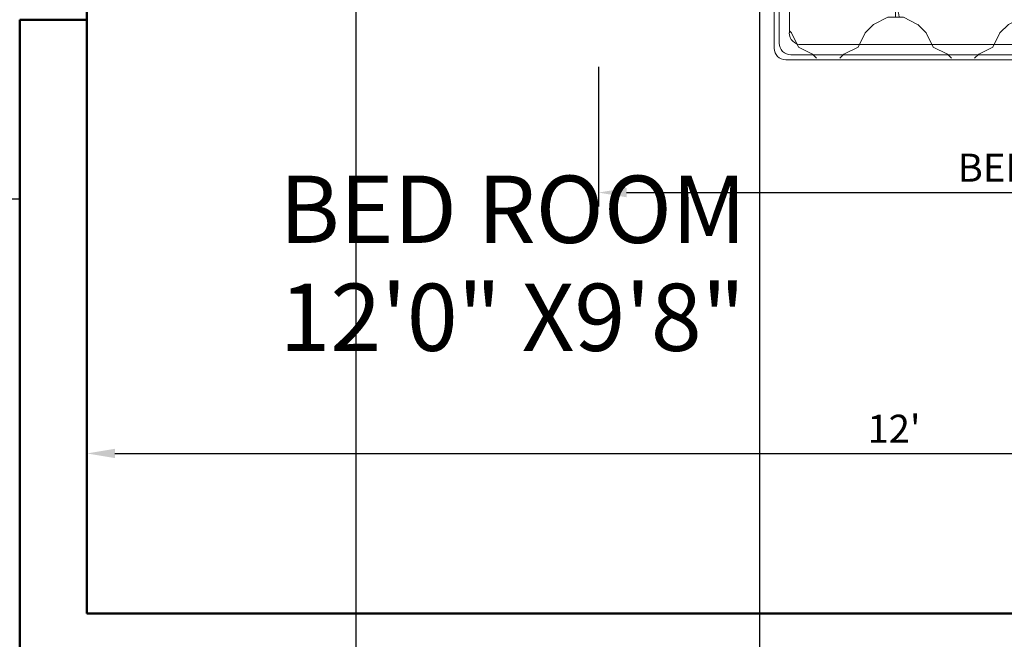
# Model space of a CAD drawing. Units: inches. Extents: x 2385 to 2740, y 1752 to 2305.
# Tile 3 of 15: x 2553 to 2641, y 1861 to 1916. Entities that reach past the tile are written whole.
import ezdxf

# ---------------------------------------------------------------- set-up
doc = ezdxf.new("R2010")
doc.units = ezdxf.units.IN
for name, color, linetype, lineweight in [('A-ANNO-DIMS', 2, 'Continuous', 18), ('A-AREA-IDEN', 7, 'Continuous', 25), ('A-FLOR-STRS', 7, 'Continuous', 25), ('A-FURN', 9, 'Continuous', 18), ('A-WALL', 7, 'Continuous', 50)]:
    doc.layers.add(name, color=color, linetype=linetype, lineweight=lineweight)
doc.styles.get("Standard").update_dxf_attribs({"font": 'arial.ttf'})
doc.dimstyles.new('Copy of ISO-25', dxfattribs={"dimtxt": 2.5, "dimasz": 2.5, "dimexe": 1.25, "dimexo": 0.625, "dimtad": 1, "dimdec": 1, "dimlunit": 4, "dimtxsty": 'Standard', "dimcen": 2.5, "dimadec": 0, "dimazin": 0, "dimtfac": 1, "dimtdec": 1, "dimtmove": 0, "dimatfit": 3, "dimfxl": 1, "dimarcsym": 0})

# ---------------------------------------------------------------- blocks, each defined once
blk = doc.blocks.new('A$C029D5C69')
for p, q in [((0.4164, 2.0693), (0.4164, 2.0066)), ((2.2315, 2.0693), (0.4164, 2.0693)), ((2.2315, 2.0066), (2.2315, 2.0693)), ((0, 1.606), (0, 2.0066)), ((0, 2.0066), (0.505, 2.0066)), ((0.4164, 2.0066), (2.2315, 2.0066)), ((0.505, 2.0066), (0.505, 1.606)), ((0.5252, 0.0351), (0.5252, 2.0066)), ((0.5403, 0.0502), (0.5403, 2.0066)), ((0.5706, 0.0805), (0.5706, 2.0066)), ((0.6869, 1.966), (0.6666, 2.0066)), ((0.7072, 2.0066), (0.6869, 1.966)), ((1.0902, 1.966), (1.0699, 2.0066)), ((1.1106, 2.0066), (1.0902, 1.966)), ((2.1114, 2.0087), (2.1114, 0.0351)), ((2.6479, 2.0066), (2.1429, 2.0066)), ((2.1429, 2.0066), (2.1429, 1.606)), ((2.6479, 1.606), (2.6479, 2.0066)), ((0.0151, 1.6211), (0.0151, 1.9915)), ((0.0151, 1.9915), (0.4899, 1.9915)), ((0.4899, 1.9915), (0.4899, 1.6211)), ((1.8954, 1.9865), (1.3081, 1.9865)), ((2.6328, 1.9915), (2.158, 1.9915)), ((2.158, 1.9915), (2.158, 1.6211)), ((2.6328, 1.6211), (2.6328, 1.9915)), ((0.2689, 1.9609), (0.2689, 1.6764)), ((0.6869, 1.9425), (0.6869, 1.966)), ((0.6869, 1.9425), (0.6869, 1.966)), ((1.0902, 1.9425), (1.0902, 1.966)), ((1.0902, 1.9425), (1.0902, 1.966)), ((1.8954, 1.9713), (1.3339, 1.9713)), ((1.3849, 1.9713), (1.3656, 1.952)), ((1.3945, 1.9713), (1.3714, 1.9483)), ((1.4249, 1.945), (1.3986, 1.9713)), ((1.4249, 1.945), (1.4059, 1.926)), ((1.4288, 1.9507), (1.4081, 1.9713)), ((1.4476, 1.9507), (1.4288, 1.9507)), ((1.4476, 1.9507), (1.4664, 1.9507)), ((1.487, 1.9713), (1.4664, 1.9507)), ((1.4966, 1.9713), (1.4703, 1.945)), ((1.4986, 1.9167), (1.4703, 1.945)), ((1.527, 1.945), (1.4986, 1.9167)), ((1.527, 1.945), (1.5007, 1.9713)), ((1.5309, 1.9507), (1.5102, 1.9713)), ((1.5497, 1.9507), (1.5309, 1.9507)), ((1.5497, 1.9507), (1.5685, 1.9507)), ((1.5891, 1.9713), (1.5685, 1.9507)), ((1.5987, 1.9713), (1.5724, 1.945)), ((1.6007, 1.9167), (1.5724, 1.945)), ((1.6291, 1.945), (1.6007, 1.9167)), ((1.6291, 1.945), (1.6028, 1.9713)), ((1.633, 1.9507), (1.6123, 1.9713)), ((1.6518, 1.9507), (1.633, 1.9507)), ((1.6518, 1.9507), (1.6706, 1.9507)), ((1.6912, 1.9713), (1.6706, 1.9507)), ((1.7008, 1.9713), (1.6745, 1.945)), ((1.7028, 1.9167), (1.6745, 1.945)), ((1.7312, 1.945), (1.7028, 1.9167)), ((1.7312, 1.945), (1.7049, 1.9713)), ((1.7351, 1.9507), (1.7144, 1.9713)), ((1.7539, 1.9507), (1.7351, 1.9507)), ((1.7539, 1.9507), (1.7727, 1.9507)), ((1.7933, 1.9713), (1.7727, 1.9507)), ((1.8029, 1.9713), (1.7766, 1.945)), ((1.8049, 1.9167), (1.7766, 1.945)), ((1.8333, 1.945), (1.8049, 1.9167)), ((1.8333, 1.945), (1.807, 1.9713)), ((1.8372, 1.9507), (1.8165, 1.9713)), ((1.856, 1.9507), (1.8372, 1.9507)), ((1.856, 1.9507), (1.8748, 1.9507)), ((1.8954, 1.9713), (1.8748, 1.9507)), ((1.9043, 1.9707), (1.8787, 1.945)), ((1.907, 1.9167), (1.8787, 1.945)), ((1.9354, 1.945), (1.907, 1.9167)), ((1.9354, 1.945), (1.9114, 1.969)), ((2.379, 1.9609), (2.379, 1.6764)), ((0.621, 1.9213), (0.5955, 1.8958)), ((0.6634, 1.9425), (0.621, 1.9213)), ((0.6634, 1.9425), (0.621, 1.9213)), ((0.6869, 1.9425), (0.6634, 1.9425)), ((0.6869, 1.9425), (0.7104, 1.9425)), ((0.7528, 1.9213), (0.7104, 1.9425)), ((0.7528, 1.9213), (0.7104, 1.9425)), ((0.7783, 1.8958), (0.7528, 1.9213)), ((1.0243, 1.9213), (0.9988, 1.8958)), ((1.0668, 1.9425), (1.0244, 1.9213)), ((1.0668, 1.9425), (1.0244, 1.9213)), ((1.0902, 1.9425), (1.0668, 1.9425)), ((1.0902, 1.9425), (1.1137, 1.9425)), ((1.1561, 1.9213), (1.1137, 1.9425)), ((1.1561, 1.9213), (1.1137, 1.9425)), ((1.1816, 1.8958), (1.1561, 1.9213)), ((1.4288, 1.9394), (1.4116, 1.9222)), ((1.4288, 1.9393), (1.4476, 1.9393)), ((1.4664, 1.9393), (1.4476, 1.9393)), ((1.493, 1.9128), (1.4664, 1.9394)), ((1.5309, 1.9394), (1.5043, 1.9128)), ((1.5309, 1.9393), (1.5497, 1.9393)), ((1.5685, 1.9393), (1.5497, 1.9393)), ((1.595, 1.9128), (1.5685, 1.9394)), ((1.633, 1.9394), (1.6064, 1.9128)), ((1.633, 1.9393), (1.6518, 1.9393)), ((1.6706, 1.9393), (1.6518, 1.9393)), ((1.6971, 1.9128), (1.6706, 1.9394)), ((1.7351, 1.9394), (1.7085, 1.9128)), ((1.7351, 1.9393), (1.7539, 1.9393)), ((1.7727, 1.9393), (1.7539, 1.9393)), ((1.7992, 1.9128), (1.7727, 1.9394)), ((1.8372, 1.9394), (1.8106, 1.9128)), ((1.8372, 1.9393), (1.856, 1.9393)), ((1.8748, 1.9393), (1.856, 1.9393)), ((1.9013, 1.9128), (1.8748, 1.9394)), ((1.9393, 1.9394), (1.9127, 1.9128)), ((1.9393, 1.9393), (1.9404, 1.9393)), ((1.9414, 1.688), (1.9414, 1.931)), ((1.9565, 1.688), (1.9565, 1.931)), ((0.5955, 1.8958), (0.5743, 1.8534)), ((0.7995, 1.8534), (0.7783, 1.8958)), ((0.9989, 1.8958), (0.9777, 1.8534)), ((1.2028, 1.8534), (1.1816, 1.8958)), ((1.493, 1.8752), (1.493, 1.9128)), ((1.5043, 1.8752), (1.5043, 1.9128)), ((1.595, 1.8752), (1.595, 1.9128)), ((1.6064, 1.8752), (1.6064, 1.9128)), ((1.6971, 1.8752), (1.6971, 1.9128)), ((1.7085, 1.8752), (1.7085, 1.9128)), ((1.7992, 1.8752), (1.7992, 1.9128)), ((1.8106, 1.8752), (1.8106, 1.9128)), ((1.9013, 1.8752), (1.9013, 1.9128)), ((1.9127, 1.8752), (1.9127, 1.9128)), ((1.493, 1.8752), (1.4867, 1.869)), ((1.4986, 1.8713), (1.4922, 1.8648)), ((1.527, 1.8429), (1.4986, 1.8713)), ((1.5309, 1.8486), (1.5043, 1.8752)), ((1.595, 1.8752), (1.5685, 1.8486)), ((1.6007, 1.8713), (1.5724, 1.8429)), ((1.6291, 1.8429), (1.6007, 1.8713)), ((1.633, 1.8486), (1.6064, 1.8752)), ((1.6971, 1.8752), (1.6706, 1.8486)), ((1.7028, 1.8713), (1.6745, 1.8429)), ((1.7312, 1.8429), (1.7028, 1.8713)), ((1.7351, 1.8486), (1.7085, 1.8752)), ((1.7992, 1.8752), (1.7727, 1.8486)), ((1.8049, 1.8713), (1.7766, 1.8429)), ((1.8333, 1.8429), (1.8049, 1.8713)), ((1.8372, 1.8486), (1.8106, 1.8752)), ((1.9013, 1.8752), (1.8748, 1.8486)), ((1.907, 1.8713), (1.8787, 1.8429)), ((1.9354, 1.8429), (1.907, 1.8713)), ((1.9393, 1.8486), (1.9127, 1.8752)), ((0.5743, 1.8534), (0.5706, 1.8515)), ((0.5743, 1.8534), (0.5706, 1.8515)), ((0.8419, 1.8322), (0.7995, 1.8534)), ((0.8419, 1.8322), (0.7995, 1.8534)), ((0.8674, 1.8067), (0.8419, 1.8322)), ((0.9352, 1.8322), (0.9097, 1.8067)), ((0.9777, 1.8534), (0.9353, 1.8322)), ((0.9777, 1.8534), (0.9353, 1.8322)), ((1.2452, 1.8322), (1.2028, 1.8534)), ((1.2452, 1.8322), (1.2028, 1.8534)), ((1.2707, 1.8067), (1.2452, 1.8322)), ((1.527, 1.8429), (1.5242, 1.8401)), ((1.5309, 1.8373), (1.5295, 1.8359)), ((1.5497, 1.8486), (1.5309, 1.8486)), ((1.5309, 1.8373), (1.5497, 1.8373)), ((1.5497, 1.8486), (1.5685, 1.8486)), ((1.5685, 1.8373), (1.5497, 1.8373)), ((1.595, 1.8107), (1.5685, 1.8373)), ((1.6007, 1.8146), (1.5724, 1.8429)), ((1.6291, 1.8429), (1.6007, 1.8146)), ((1.633, 1.8373), (1.6064, 1.8107)), ((1.6518, 1.8486), (1.633, 1.8486)), ((1.633, 1.8373), (1.6518, 1.8373)), ((1.6518, 1.8486), (1.6706, 1.8486)), ((1.6706, 1.8373), (1.6518, 1.8373)), ((1.6971, 1.8107), (1.6706, 1.8373)), ((1.7028, 1.8146), (1.6745, 1.8429)), ((1.7312, 1.8429), (1.7028, 1.8146)), ((1.7351, 1.8373), (1.7085, 1.8107)), ((1.7539, 1.8486), (1.7351, 1.8486)), ((1.7351, 1.8373), (1.7539, 1.8373)), ((1.7539, 1.8486), (1.7727, 1.8486)), ((1.7727, 1.8373), (1.7539, 1.8373)), ((1.7992, 1.8107), (1.7727, 1.8373)), ((1.8049, 1.8146), (1.7766, 1.8429)), ((1.8333, 1.8429), (1.8049, 1.8146)), ((1.8372, 1.8373), (1.8106, 1.8107)), ((1.856, 1.8486), (1.8372, 1.8486)), ((1.8372, 1.8373), (1.856, 1.8373)), ((1.856, 1.8486), (1.8748, 1.8486)), ((1.8748, 1.8373), (1.856, 1.8373)), ((1.9013, 1.8107), (1.8748, 1.8373)), ((1.907, 1.8146), (1.8787, 1.8429)), ((1.9354, 1.8429), (1.907, 1.8146)), ((1.9393, 1.8373), (1.9127, 1.8107)), ((1.9414, 1.8486), (1.9393, 1.8486)), ((1.9393, 1.8373), (1.9414, 1.8373)), ((0.1267, 1.8186), (0.4111, 1.8186)), ((0.8886, 1.7643), (0.8674, 1.8067)), ((0.9098, 1.8067), (0.8886, 1.7643)), ((1.2919, 1.7643), (1.2707, 1.8067)), ((1.595, 1.7806), (1.595, 1.8107)), ((1.6064, 1.7731), (1.6064, 1.8107)), ((1.6971, 1.7731), (1.6971, 1.8107)), ((1.7085, 1.7731), (1.7085, 1.8107)), ((1.7992, 1.7731), (1.7992, 1.8107)), ((1.8106, 1.7731), (1.8106, 1.8107)), ((1.9013, 1.7731), (1.9013, 1.8107)), ((1.9127, 1.7731), (1.9127, 1.8107)), ((2.2367, 1.8186), (2.5212, 1.8186)), ((1.2981, 1.7768), (1.2919, 1.7643)), ((1.633, 1.7465), (1.6064, 1.7731)), ((1.6971, 1.7731), (1.6706, 1.7465)), ((1.7028, 1.7692), (1.6745, 1.7408)), ((1.7312, 1.7408), (1.7028, 1.7692)), ((1.7351, 1.7465), (1.7085, 1.7731)), ((1.7992, 1.7731), (1.7727, 1.7465)), ((1.8049, 1.7692), (1.7766, 1.7408)), ((1.8333, 1.7408), (1.8049, 1.7692)), ((1.8372, 1.7465), (1.8106, 1.7731)), ((1.9013, 1.7731), (1.8748, 1.7465)), ((1.907, 1.7692), (1.8787, 1.7408)), ((1.9354, 1.7408), (1.907, 1.7692)), ((1.9393, 1.7465), (1.9127, 1.7731)), ((0.8651, 1.7408), (0.8227, 1.7196)), ((0.8651, 1.7408), (0.8227, 1.7196)), ((0.912, 1.7408), (0.8651, 1.7408)), ((0.8886, 1.7408), (0.8886, 1.7643)), ((0.9544, 1.7196), (0.912, 1.7408)), ((0.9544, 1.7196), (0.912, 1.7408)), ((1.2684, 1.7408), (1.226, 1.7196)), ((1.2684, 1.7408), (1.226, 1.7196)), ((1.2885, 1.7408), (1.2684, 1.7408)), ((1.2919, 1.7519), (1.2919, 1.7643)), ((1.6518, 1.7465), (1.633, 1.7465)), ((1.6518, 1.7465), (1.6706, 1.7465)), ((1.7028, 1.7125), (1.6745, 1.7408)), ((1.7312, 1.7408), (1.7028, 1.7125)), ((1.7539, 1.7465), (1.7351, 1.7465)), ((1.7539, 1.7465), (1.7727, 1.7465)), ((1.8049, 1.7125), (1.7766, 1.7408)), ((1.8333, 1.7408), (1.8049, 1.7125)), ((1.856, 1.7465), (1.8372, 1.7465)), ((1.856, 1.7465), (1.8748, 1.7465)), ((1.907, 1.7125), (1.8787, 1.7408)), ((1.9354, 1.7408), (1.907, 1.7125)), ((1.9414, 1.7465), (1.9393, 1.7465)), ((0.8227, 1.7196), (0.7972, 1.6941)), ((0.98, 1.6941), (0.9545, 1.7196)), ((1.226, 1.7196), (1.2005, 1.6941)), ((1.6443, 1.7352), (1.6518, 1.7352)), ((1.6706, 1.7352), (1.6518, 1.7352)), ((1.6971, 1.7086), (1.6706, 1.7352)), ((1.6971, 1.682), (1.6971, 1.7086)), ((1.7351, 1.7352), (1.7085, 1.7086)), ((1.7085, 1.671), (1.7085, 1.7086)), ((1.7351, 1.7352), (1.7539, 1.7352)), ((1.7727, 1.7352), (1.7539, 1.7352)), ((1.7992, 1.7086), (1.7727, 1.7352)), ((1.7992, 1.671), (1.7992, 1.7086)), ((1.8372, 1.7352), (1.8106, 1.7086)), ((1.8106, 1.671), (1.8106, 1.7086)), ((1.8372, 1.7352), (1.856, 1.7352)), ((1.8748, 1.7352), (1.856, 1.7352)), ((1.9013, 1.7086), (1.8748, 1.7352)), ((1.9013, 1.671), (1.9013, 1.7086)), ((1.9393, 1.7352), (1.9127, 1.7086)), ((1.9127, 1.671), (1.9127, 1.7086)), ((1.9393, 1.7352), (1.9414, 1.7352)), ((0.5766, 1.6941), (0.5706, 1.7002)), ((0.5978, 1.6517), (0.5766, 1.6941)), ((0.7972, 1.6941), (0.776, 1.6517)), ((1.0011, 1.6517), (0.9799, 1.6941)), ((1.2005, 1.6941), (1.1793, 1.6517)), ((2.5551, 1.6275), (2.5551, 1.696)), ((0.6402, 1.6305), (0.5978, 1.6517)), ((0.6402, 1.6305), (0.5978, 1.6517)), ((0.776, 1.6517), (0.7336, 1.6305)), ((0.776, 1.6517), (0.7336, 1.6305)), ((1.0435, 1.6305), (1.0011, 1.6517)), ((1.0435, 1.6305), (1.0011, 1.6517)), ((1.1793, 1.6517), (1.1369, 1.6305)), ((1.1793, 1.6517), (1.1369, 1.6305)), ((1.7318, 1.6477), (1.7085, 1.671)), ((1.7992, 1.671), (1.7759, 1.6477)), ((1.8049, 1.6671), (1.7855, 1.6477)), ((1.8244, 1.6477), (1.8049, 1.6671)), ((1.8339, 1.6477), (1.8106, 1.671)), ((1.9013, 1.671), (1.878, 1.6477)), ((1.907, 1.6671), (1.8876, 1.6477)), ((1.9202, 1.6539), (1.907, 1.6671)), ((1.926, 1.6577), (1.9127, 1.671)), ((0.4899, 1.6211), (0.0151, 1.6211)), ((0.6657, 1.605), (0.6402, 1.6305)), ((0.7336, 1.6305), (0.7081, 1.605)), ((1.0691, 1.605), (1.0436, 1.6305)), ((1.1369, 1.6305), (1.1114, 1.605)), ((1.8961, 1.6477), (1.7289, 1.6477)), ((1.8961, 1.6325), (1.7422, 1.6325)), ((2.158, 1.6211), (2.6328, 1.6211)), ((0.505, 1.606), (0, 1.606)), ((0.6869, 1.5626), (0.6657, 1.605)), ((0.7081, 1.605), (0.6869, 1.5626)), ((1.0902, 1.5626), (1.069, 1.605)), ((1.1114, 1.605), (1.0902, 1.5626)), ((2.1429, 1.606), (2.6479, 1.606)), ((0.6869, 1.5392), (0.6869, 1.5626)), ((0.6869, 1.5392), (0.6869, 1.5626)), ((1.0902, 1.5392), (1.0902, 1.5626)), ((1.0902, 1.5392), (1.0902, 1.5626)), ((0.6634, 1.5391), (0.621, 1.5179)), ((0.6634, 1.5391), (0.621, 1.5179)), ((0.6869, 1.5392), (0.6634, 1.5392)), ((0.6869, 1.5392), (0.7104, 1.5392)), ((0.7528, 1.5179), (0.7104, 1.5391)), ((0.7528, 1.5179), (0.7104, 1.5391)), ((1.0668, 1.5391), (1.0244, 1.5179)), ((1.0668, 1.5391), (1.0244, 1.5179)), ((1.0902, 1.5392), (1.0668, 1.5392)), ((1.0902, 1.5392), (1.1137, 1.5392)), ((1.1561, 1.5179), (1.1137, 1.5391)), ((1.1561, 1.5179), (1.1137, 1.5391)), ((0.621, 1.5179), (0.5955, 1.4924)), ((0.7783, 1.4924), (0.7528, 1.5179)), ((1.0243, 1.5179), (0.9988, 1.4924)), ((1.1816, 1.4924), (1.1561, 1.5179)), ((1.4277, 1.5179), (1.4022, 1.4924)), ((1.4534, 1.5308), (1.4277, 1.5179)), ((1.4534, 1.5308), (1.4277, 1.5179)), ((0.5955, 1.4925), (0.5743, 1.4501)), ((0.7995, 1.4501), (0.7783, 1.4925)), ((0.9989, 1.4925), (0.9777, 1.4501)), ((1.2028, 1.4501), (1.1816, 1.4925)), ((1.4022, 1.4925), (1.381, 1.4501)), ((0.5743, 1.45), (0.5706, 1.4481)), ((0.5743, 1.45), (0.5706, 1.4481)), ((0.8419, 1.4288), (0.7995, 1.45)), ((0.8419, 1.4288), (0.7995, 1.45)), ((0.9777, 1.45), (0.9353, 1.4288)), ((0.9777, 1.45), (0.9353, 1.4288)), ((1.2452, 1.4288), (1.2028, 1.45)), ((1.2452, 1.4288), (1.2028, 1.45)), ((1.381, 1.45), (1.3386, 1.4288)), ((1.381, 1.45), (1.3386, 1.4288)), ((1.6062, 1.4501), (1.5966, 1.4692)), ((1.6486, 1.4288), (1.6062, 1.45)), ((1.6486, 1.4288), (1.6062, 1.45)), ((0.8674, 1.4033), (0.8419, 1.4288)), ((0.9352, 1.4288), (0.9097, 1.4033)), ((1.2707, 1.4033), (1.2452, 1.4288)), ((1.3386, 1.4288), (1.3131, 1.4033)), ((1.6741, 1.4033), (1.6486, 1.4288)), ((0.5403, 1.4117), (0.5706, 1.4117)), ((0.8886, 1.361), (0.8674, 1.4034)), ((0.9098, 1.4034), (0.8886, 1.361)), ((1.2919, 1.361), (1.2707, 1.4034)), ((1.3131, 1.4034), (1.2919, 1.361)), ((1.6953, 1.361), (1.6741, 1.4034)), ((1.714, 1.3984), (1.6953, 1.361)), ((0.8886, 1.3375), (0.8886, 1.3609)), ((1.2919, 1.3375), (1.2919, 1.3609)), ((1.6953, 1.3375), (1.6953, 1.3609)), ((0.8651, 1.3374), (0.8227, 1.3162)), ((0.8651, 1.3374), (0.8227, 1.3162)), ((0.912, 1.3375), (0.8651, 1.3375)), ((0.9544, 1.3162), (0.912, 1.3374)), ((0.9544, 1.3162), (0.912, 1.3374)), ((1.2684, 1.3374), (1.226, 1.3162)), ((1.2684, 1.3374), (1.226, 1.3162)), ((1.3154, 1.3375), (1.2684, 1.3375)), ((1.3578, 1.3162), (1.3154, 1.3374)), ((1.3578, 1.3162), (1.3154, 1.3374)), ((1.6718, 1.3374), (1.6294, 1.3162)), ((1.6718, 1.3374), (1.6294, 1.3162)), ((1.7187, 1.3375), (1.6718, 1.3375)), ((1.7611, 1.3162), (1.7187, 1.3374)), ((1.7611, 1.3162), (1.7187, 1.3374)), ((0.5766, 1.2908), (0.5706, 1.2968)), ((0.8227, 1.3163), (0.7972, 1.2908)), ((0.98, 1.2908), (0.9545, 1.3163)), ((1.226, 1.3163), (1.2005, 1.2908)), ((1.3833, 1.2908), (1.3578, 1.3163)), ((1.6294, 1.3163), (1.6039, 1.2908)), ((1.7867, 1.2908), (1.7611, 1.3163)), ((0.5978, 1.2484), (0.5766, 1.2908)), ((0.7972, 1.2908), (0.776, 1.2484)), ((1.0011, 1.2484), (0.9799, 1.2908)), ((1.2005, 1.2908), (1.1793, 1.2484)), ((1.4045, 1.2484), (1.3833, 1.2908)), ((1.6039, 1.2908), (1.5827, 1.2484)), ((1.8078, 1.2484), (1.7866, 1.2908)), ((0.6402, 1.2271), (0.5978, 1.2483)), ((0.6402, 1.2271), (0.5978, 1.2483)), ((0.776, 1.2483), (0.7336, 1.2271)), ((0.776, 1.2483), (0.7336, 1.2271)), ((1.0435, 1.2271), (1.0011, 1.2483)), ((1.0435, 1.2271), (1.0011, 1.2483)), ((1.1793, 1.2483), (1.1369, 1.2271)), ((1.1793, 1.2483), (1.1369, 1.2271)), ((1.4469, 1.2271), (1.4045, 1.2483)), ((1.4469, 1.2271), (1.4045, 1.2483)), ((1.5827, 1.2483), (1.5403, 1.2271)), ((1.5827, 1.2483), (1.5403, 1.2271)), ((1.8502, 1.2271), (1.8078, 1.2483)), ((1.8502, 1.2271), (1.8078, 1.2483)), ((0.5403, 1.21), (0.5706, 1.21)), ((0.6657, 1.2017), (0.6402, 1.2272)), ((0.7336, 1.2272), (0.7081, 1.2017)), ((1.0691, 1.2017), (1.0436, 1.2272)), ((1.1369, 1.2272), (1.1114, 1.2017)), ((1.4724, 1.2017), (1.4469, 1.2272)), ((1.5403, 1.2272), (1.5148, 1.2017)), ((1.8758, 1.2017), (1.8503, 1.2272)), ((0.6869, 1.1593), (0.6657, 1.2017)), ((0.7081, 1.2017), (0.6869, 1.1593)), ((1.0902, 1.1593), (1.069, 1.2017)), ((1.1114, 1.2017), (1.0902, 1.1593)), ((1.4936, 1.1593), (1.4724, 1.2017)), ((1.5148, 1.2017), (1.4936, 1.1593)), ((1.8969, 1.1593), (1.8757, 1.2017)), ((1.9181, 1.2017), (1.8969, 1.1593)), ((1.9215, 1.2051), (1.9181, 1.2017)), ((0.6869, 1.1358), (0.6869, 1.1593)), ((0.6869, 1.1358), (0.6869, 1.1593)), ((1.0902, 1.1358), (1.0902, 1.1593)), ((1.0902, 1.1358), (1.0902, 1.1593)), ((1.4936, 1.1358), (1.4936, 1.1593)), ((1.4936, 1.1358), (1.4936, 1.1593)), ((1.8969, 1.1358), (1.8969, 1.1593)), ((1.8969, 1.1358), (1.8969, 1.1593)), ((0.6634, 1.1358), (0.621, 1.1146)), ((0.6634, 1.1358), (0.621, 1.1146)), ((0.6869, 1.1358), (0.6634, 1.1358)), ((0.6869, 1.1358), (0.7104, 1.1358)), ((0.7528, 1.1146), (0.7104, 1.1358)), ((0.7528, 1.1146), (0.7104, 1.1358)), ((1.0668, 1.1358), (1.0244, 1.1146)), ((1.0668, 1.1358), (1.0244, 1.1146)), ((1.0902, 1.1358), (1.0668, 1.1358)), ((1.0902, 1.1358), (1.1137, 1.1358)), ((1.1561, 1.1146), (1.1137, 1.1358)), ((1.1561, 1.1146), (1.1137, 1.1358)), ((1.4701, 1.1358), (1.4277, 1.1146)), ((1.4701, 1.1358), (1.4277, 1.1146)), ((1.4936, 1.1358), (1.4701, 1.1358)), ((1.4936, 1.1358), (1.5171, 1.1358)), ((1.5595, 1.1146), (1.5171, 1.1358)), ((1.5595, 1.1146), (1.5171, 1.1358)), ((1.8735, 1.1358), (1.8311, 1.1146)), ((1.8735, 1.1358), (1.8311, 1.1146)), ((1.8969, 1.1358), (1.8735, 1.1358)), ((1.8969, 1.1358), (1.9204, 1.1358)), ((1.9628, 1.1146), (1.9204, 1.1358)), ((1.9628, 1.1146), (1.9204, 1.1358)), ((0.621, 1.1146), (0.5955, 1.0891)), ((0.7783, 1.0891), (0.7528, 1.1146)), ((1.0243, 1.1146), (0.9988, 1.0891)), ((1.1816, 1.0891), (1.1561, 1.1146)), ((1.4277, 1.1146), (1.4022, 1.0891)), ((1.585, 1.0891), (1.5595, 1.1146)), ((1.831, 1.1146), (1.8055, 1.0891)), ((1.9883, 1.0891), (1.9628, 1.1146)), ((0.5955, 1.0891), (0.5743, 1.0467)), ((0.7995, 1.0467), (0.7783, 1.0891)), ((0.9989, 1.0891), (0.9777, 1.0467)), ((1.2028, 1.0467), (1.1816, 1.0891)), ((1.4022, 1.0891), (1.381, 1.0467)), ((1.6062, 1.0467), (1.585, 1.0891)), ((1.8056, 1.0891), (1.7844, 1.0467)), ((2.0095, 1.0467), (1.9883, 1.0891)), ((0.5743, 1.0467), (0.5706, 1.0448)), ((0.5743, 1.0467), (0.5706, 1.0448)), ((0.8419, 1.0255), (0.7995, 1.0467)), ((0.8419, 1.0255), (0.7995, 1.0467)), ((0.9777, 1.0467), (0.9353, 1.0255)), ((0.9777, 1.0467), (0.9353, 1.0255)), ((1.2452, 1.0255), (1.2028, 1.0467)), ((1.2452, 1.0255), (1.2028, 1.0467)), ((1.381, 1.0467), (1.3386, 1.0255)), ((1.381, 1.0467), (1.3386, 1.0255)), ((1.6486, 1.0255), (1.6062, 1.0467)), ((1.6486, 1.0255), (1.6062, 1.0467)), ((1.7844, 1.0467), (1.742, 1.0255)), ((1.7844, 1.0467), (1.742, 1.0255)), ((2.0276, 1.0376), (2.0095, 1.0467)), ((2.0276, 1.0376), (2.0095, 1.0467)), ((0.8674, 1), (0.8419, 1.0255)), ((0.9352, 1.0255), (0.9097, 1)), ((1.2707, 1), (1.2452, 1.0255)), ((1.3386, 1.0255), (1.3131, 1)), ((1.6741, 1), (1.6486, 1.0255)), ((1.7419, 1.0255), (1.7164, 1)), ((0.8886, 0.9576), (0.8674, 1)), ((0.9098, 1), (0.8886, 0.9576)), ((1.2919, 0.9576), (1.2707, 1)), ((1.3131, 1), (1.2919, 0.9576)), ((1.6953, 0.9576), (1.6741, 1)), ((1.7165, 1), (1.6953, 0.9576)), ((0.8886, 0.9341), (0.8886, 0.9576)), ((1.2919, 0.9341), (1.2919, 0.9576)), ((1.6953, 0.9341), (1.6953, 0.9576)), ((2.066, 0.9457), (2.066, 0.0805)), ((0.8651, 0.9341), (0.8227, 0.9129)), ((0.8651, 0.9341), (0.8227, 0.9129)), ((0.912, 0.9341), (0.8651, 0.9341)), ((0.9544, 0.9129), (0.912, 0.9341)), ((0.9544, 0.9129), (0.912, 0.9341)), ((1.2684, 0.9341), (1.226, 0.9129)), ((1.2684, 0.9341), (1.226, 0.9129)), ((1.3154, 0.9341), (1.2684, 0.9341)), ((1.3578, 0.9129), (1.3154, 0.9341)), ((1.3578, 0.9129), (1.3154, 0.9341)), ((1.6718, 0.9341), (1.6294, 0.9129)), ((1.6718, 0.9341), (1.6294, 0.9129)), ((1.7187, 0.9341), (1.6718, 0.9341)), ((1.7611, 0.9129), (1.7187, 0.9341)), ((1.7611, 0.9129), (1.7187, 0.9341)), ((2.066, 0.9295), (2.0327, 0.9129)), ((2.066, 0.9295), (2.0327, 0.9129)), ((0.5766, 0.8874), (0.5706, 0.8935)), ((0.5978, 0.845), (0.5766, 0.8874)), ((0.7972, 0.8874), (0.776, 0.845)), ((0.8227, 0.9129), (0.7972, 0.8874)), ((0.98, 0.8874), (0.9545, 0.9129)), ((1.0011, 0.845), (0.9799, 0.8874)), ((1.2005, 0.8874), (1.1793, 0.845)), ((1.226, 0.9129), (1.2005, 0.8874)), ((1.3833, 0.8874), (1.3578, 0.9129)), ((1.4045, 0.845), (1.3833, 0.8874)), ((1.6039, 0.8874), (1.5827, 0.845)), ((1.6294, 0.9129), (1.6039, 0.8874)), ((1.7867, 0.8874), (1.7611, 0.9129)), ((1.8078, 0.845), (1.7866, 0.8874)), ((2.0072, 0.8874), (1.986, 0.845)), ((2.0327, 0.9129), (2.0072, 0.8874)), ((0.6402, 0.8238), (0.5978, 0.845)), ((0.6402, 0.8238), (0.5978, 0.845)), ((0.776, 0.845), (0.7336, 0.8238)), ((0.776, 0.845), (0.7336, 0.8238)), ((1.0435, 0.8238), (1.0011, 0.845)), ((1.0435, 0.8238), (1.0011, 0.845)), ((1.1793, 0.845), (1.1369, 0.8238)), ((1.1793, 0.845), (1.1369, 0.8238)), ((1.4469, 0.8238), (1.4045, 0.845)), ((1.4469, 0.8238), (1.4045, 0.845)), ((1.5827, 0.845), (1.5403, 0.8238)), ((1.5827, 0.845), (1.5403, 0.8238)), ((1.8502, 0.8238), (1.8078, 0.845)), ((1.8502, 0.8238), (1.8078, 0.845)), ((1.986, 0.845), (1.9436, 0.8238)), ((1.986, 0.845), (1.9436, 0.8238)), ((2.0962, 0.8369), (2.0962, 0.0502)), ((0.6657, 0.7983), (0.6402, 0.8238)), ((0.6869, 0.7559), (0.6657, 0.7983)), ((0.7081, 0.7983), (0.6869, 0.7559)), ((0.7336, 0.8238), (0.7081, 0.7983)), ((1.0691, 0.7983), (1.0436, 0.8238)), ((1.0902, 0.7559), (1.069, 0.7983)), ((1.1114, 0.7983), (1.0902, 0.7559)), ((1.1369, 0.8238), (1.1114, 0.7983)), ((1.4724, 0.7983), (1.4469, 0.8238)), ((1.4936, 0.7559), (1.4724, 0.7983)), ((1.5148, 0.7983), (1.4936, 0.7559)), ((1.5403, 0.8238), (1.5148, 0.7983)), ((1.8758, 0.7983), (1.8503, 0.8238)), ((1.8969, 0.7559), (1.8757, 0.7983)), ((1.9181, 0.7983), (1.8969, 0.7559)), ((1.9436, 0.8238), (1.9181, 0.7983)), ((0.6869, 0.7325), (0.6869, 0.7559)), ((0.6869, 0.7325), (0.6869, 0.7559)), ((1.0902, 0.7325), (1.0902, 0.7559)), ((1.0902, 0.7325), (1.0902, 0.7559)), ((1.2024, 0.7028), (1.2503, 0.7507)), ((1.4936, 0.7325), (1.4936, 0.7559)), ((1.4936, 0.7325), (1.4936, 0.7559)), ((1.8969, 0.7325), (1.8969, 0.7559)), ((1.8969, 0.7325), (1.8969, 0.7559)), ((0.621, 0.7113), (0.5955, 0.6858)), ((0.6634, 0.7324), (0.621, 0.7112)), ((0.6634, 0.7324), (0.621, 0.7112)), ((0.6869, 0.7325), (0.6634, 0.7325)), ((0.6869, 0.7325), (0.7104, 0.7325)), ((0.7528, 0.7112), (0.7104, 0.7324)), ((0.7528, 0.7112), (0.7104, 0.7324)), ((0.7783, 0.6858), (0.7528, 0.7113)), ((1.0243, 0.7113), (0.9988, 0.6858)), ((1.0668, 0.7324), (1.0244, 0.7112)), ((1.0668, 0.7324), (1.0244, 0.7112)), ((1.0902, 0.7325), (1.0668, 0.7325)), ((1.0902, 0.7325), (1.1137, 0.7325)), ((1.1561, 0.7112), (1.1137, 0.7324)), ((1.1561, 0.7112), (1.1137, 0.7324)), ((1.1816, 0.6858), (1.1561, 0.7113)), ((1.4277, 0.7113), (1.4022, 0.6858)), ((1.4701, 0.7324), (1.4277, 0.7112)), ((1.4701, 0.7324), (1.4277, 0.7112)), ((1.4936, 0.7325), (1.4701, 0.7325)), ((1.4936, 0.7325), (1.5171, 0.7325)), ((1.5595, 0.7112), (1.5171, 0.7324)), ((1.5595, 0.7112), (1.5171, 0.7324)), ((1.585, 0.6858), (1.5595, 0.7113)), ((1.831, 0.7113), (1.8055, 0.6858)), ((1.8735, 0.7324), (1.8311, 0.7112)), ((1.8735, 0.7324), (1.8311, 0.7112)), ((1.8969, 0.7325), (1.8735, 0.7325)), ((1.8969, 0.7325), (1.9204, 0.7325)), ((1.9628, 0.7112), (1.9204, 0.7324)), ((1.9628, 0.7112), (1.9204, 0.7324)), ((1.9883, 0.6858), (1.9628, 0.7113)), ((0.5955, 0.6858), (0.5743, 0.6434)), ((0.7995, 0.6434), (0.7783, 0.6858)), ((0.9989, 0.6858), (0.9777, 0.6434)), ((1.2028, 0.6434), (1.1816, 0.6858)), ((1.4022, 0.6858), (1.381, 0.6434)), ((1.6062, 0.6434), (1.585, 0.6858)), ((1.8056, 0.6858), (1.7844, 0.6434)), ((2.0095, 0.6434), (1.9883, 0.6858)), ((0.5743, 0.6433), (0.5706, 0.6414)), ((0.5743, 0.6433), (0.5706, 0.6414)), ((0.8419, 0.6221), (0.7995, 0.6433)), ((0.8419, 0.6221), (0.7995, 0.6433)), ((0.8674, 0.5967), (0.8419, 0.6222)), ((0.9352, 0.6222), (0.9097, 0.5967)), ((0.9777, 0.6433), (0.9353, 0.6221)), ((0.9777, 0.6433), (0.9353, 0.6221)), ((1.2452, 0.6221), (1.2028, 0.6433)), ((1.2452, 0.6221), (1.2028, 0.6433)), ((1.2707, 0.5967), (1.2452, 0.6222)), ((1.3386, 0.6222), (1.3131, 0.5967)), ((1.381, 0.6433), (1.3386, 0.6221)), ((1.381, 0.6433), (1.3386, 0.6221)), ((1.6486, 0.6221), (1.6062, 0.6433)), ((1.6486, 0.6221), (1.6062, 0.6433)), ((1.6741, 0.5967), (1.6486, 0.6222)), ((1.7419, 0.6222), (1.7164, 0.5967)), ((1.7844, 0.6433), (1.742, 0.6221)), ((1.7844, 0.6433), (1.742, 0.6221)), ((2.0519, 0.6221), (2.0095, 0.6433)), ((2.0519, 0.6221), (2.0095, 0.6433)), ((2.066, 0.6081), (2.0519, 0.6222)), ((0.8886, 0.5543), (0.8674, 0.5967)), ((0.9098, 0.5967), (0.8886, 0.5543)), ((1.2919, 0.5543), (1.2707, 0.5967)), ((1.3131, 0.5967), (1.2919, 0.5543)), ((1.6953, 0.5543), (1.6741, 0.5967)), ((1.7165, 0.5967), (1.6953, 0.5543)), ((0.8651, 0.5308), (0.8227, 0.5096)), ((0.8651, 0.5308), (0.8227, 0.5096)), ((0.912, 0.5308), (0.8651, 0.5308)), ((0.8886, 0.5308), (0.8886, 0.5543)), ((0.9544, 0.5096), (0.912, 0.5308)), ((0.9544, 0.5096), (0.912, 0.5308)), ((1.2684, 0.5308), (1.226, 0.5096)), ((1.2684, 0.5308), (1.226, 0.5096)), ((1.3154, 0.5308), (1.2684, 0.5308)), ((1.2919, 0.5308), (1.2919, 0.5543)), ((1.3578, 0.5096), (1.3154, 0.5308)), ((1.3578, 0.5096), (1.3154, 0.5308)), ((1.6718, 0.5308), (1.6294, 0.5096)), ((1.6718, 0.5308), (1.6294, 0.5096)), ((1.7187, 0.5308), (1.6718, 0.5308)), ((1.6953, 0.5308), (1.6953, 0.5543)), ((1.7611, 0.5096), (1.7187, 0.5308)), ((1.7611, 0.5096), (1.7187, 0.5308)), ((0.8227, 0.5096), (0.7972, 0.4841)), ((0.98, 0.4841), (0.9545, 0.5096)), ((1.226, 0.5096), (1.2005, 0.4841)), ((1.3833, 0.4841), (1.3578, 0.5096)), ((1.6294, 0.5096), (1.6039, 0.4841)), ((1.7867, 0.4841), (1.7611, 0.5096)), ((2.0327, 0.5096), (2.0072, 0.4841)), ((2.066, 0.5262), (2.0327, 0.5096)), ((2.066, 0.5262), (2.0327, 0.5096)), ((0.5766, 0.4841), (0.5706, 0.4901)), ((0.5978, 0.4417), (0.5766, 0.4841)), ((0.7972, 0.4841), (0.776, 0.4417)), ((1.0011, 0.4417), (0.9799, 0.4841)), ((1.2005, 0.4841), (1.1793, 0.4417)), ((1.4045, 0.4417), (1.3833, 0.4841)), ((1.6039, 0.4841), (1.5827, 0.4417)), ((1.8078, 0.4417), (1.7866, 0.4841)), ((2.0072, 0.4841), (1.986, 0.4417)), ((0.6402, 0.4205), (0.5978, 0.4417)), ((0.6402, 0.4205), (0.5978, 0.4417)), ((0.6657, 0.395), (0.6402, 0.4205)), ((0.7336, 0.4205), (0.7081, 0.395)), ((0.776, 0.4417), (0.7336, 0.4205)), ((0.776, 0.4417), (0.7336, 0.4205)), ((1.0435, 0.4205), (1.0011, 0.4417)), ((1.0435, 0.4205), (1.0011, 0.4417)), ((1.0691, 0.395), (1.0436, 0.4205)), ((1.1369, 0.4205), (1.1114, 0.395)), ((1.1793, 0.4417), (1.1369, 0.4205)), ((1.1793, 0.4417), (1.1369, 0.4205)), ((1.4469, 0.4205), (1.4045, 0.4417)), ((1.4469, 0.4205), (1.4045, 0.4417)), ((1.4724, 0.395), (1.4469, 0.4205)), ((1.5403, 0.4205), (1.5148, 0.395)), ((1.5827, 0.4417), (1.5403, 0.4205)), ((1.5827, 0.4417), (1.5403, 0.4205)), ((1.8502, 0.4205), (1.8078, 0.4417)), ((1.8502, 0.4205), (1.8078, 0.4417)), ((1.8758, 0.395), (1.8503, 0.4205)), ((1.9436, 0.4205), (1.9181, 0.395)), ((1.986, 0.4417), (1.9436, 0.4205)), ((1.986, 0.4417), (1.9436, 0.4205)), ((0.6869, 0.3526), (0.6657, 0.395)), ((0.7081, 0.395), (0.6869, 0.3526)), ((1.0902, 0.3526), (1.069, 0.395)), ((1.1114, 0.395), (1.0902, 0.3526)), ((1.4936, 0.3526), (1.4724, 0.395)), ((1.5148, 0.395), (1.4936, 0.3526)), ((1.8969, 0.3526), (1.8757, 0.395)), ((1.9181, 0.395), (1.8969, 0.3526)), ((0.6634, 0.3291), (0.621, 0.3079)), ((0.6634, 0.3291), (0.621, 0.3079)), ((0.6869, 0.3291), (0.6634, 0.3291)), ((0.6869, 0.3291), (0.6869, 0.3526)), ((0.6869, 0.3291), (0.6869, 0.3526)), ((0.6869, 0.3291), (0.7104, 0.3291)), ((0.7528, 0.3079), (0.7104, 0.3291)), ((0.7528, 0.3079), (0.7104, 0.3291)), ((1.0668, 0.3291), (1.0244, 0.3079)), ((1.0668, 0.3291), (1.0244, 0.3079)), ((1.0902, 0.3291), (1.0668, 0.3291)), ((1.0902, 0.3291), (1.0902, 0.3526)), ((1.0902, 0.3291), (1.0902, 0.3526)), ((1.0902, 0.3291), (1.1137, 0.3291)), ((1.1561, 0.3079), (1.1137, 0.3291)), ((1.1561, 0.3079), (1.1137, 0.3291)), ((1.4701, 0.3291), (1.4277, 0.3079)), ((1.4701, 0.3291), (1.4277, 0.3079)), ((1.4936, 0.3291), (1.4701, 0.3291)), ((1.4936, 0.3291), (1.4936, 0.3526)), ((1.4936, 0.3291), (1.4936, 0.3526)), ((1.4936, 0.3291), (1.5171, 0.3291)), ((1.5595, 0.3079), (1.5171, 0.3291)), ((1.5595, 0.3079), (1.5171, 0.3291)), ((1.8735, 0.3291), (1.8311, 0.3079)), ((1.8735, 0.3291), (1.8311, 0.3079)), ((1.8969, 0.3291), (1.8735, 0.3291)), ((1.8969, 0.3291), (1.8969, 0.3526)), ((1.8969, 0.3291), (1.8969, 0.3526)), ((1.8969, 0.3291), (1.9204, 0.3291)), ((1.9628, 0.3079), (1.9204, 0.3291)), ((1.9628, 0.3079), (1.9204, 0.3291)), ((0.621, 0.3079), (0.5955, 0.2824)), ((0.7783, 0.2824), (0.7528, 0.3079)), ((1.0243, 0.3079), (0.9988, 0.2824)), ((1.1816, 0.2824), (1.1561, 0.3079)), ((1.4277, 0.3079), (1.4022, 0.2824)), ((1.585, 0.2824), (1.5595, 0.3079)), ((1.831, 0.3079), (1.8055, 0.2824)), ((1.9883, 0.2824), (1.9628, 0.3079)), ((0.5955, 0.2824), (0.5743, 0.24)), ((0.7995, 0.24), (0.7783, 0.2824)), ((0.9989, 0.2824), (0.9777, 0.24)), ((1.2028, 0.24), (1.1816, 0.2824)), ((1.4022, 0.2824), (1.381, 0.24)), ((1.6062, 0.24), (1.585, 0.2824)), ((1.8056, 0.2824), (1.7844, 0.24)), ((2.0095, 0.24), (1.9883, 0.2824)), ((0.5743, 0.24), (0.5706, 0.2381)), ((0.5743, 0.24), (0.5706, 0.2381)), ((0.8419, 0.2188), (0.7995, 0.24)), ((0.8419, 0.2188), (0.7995, 0.24)), ((0.9777, 0.24), (0.9353, 0.2188)), ((0.9777, 0.24), (0.9353, 0.2188)), ((1.2452, 0.2188), (1.2028, 0.24)), ((1.2452, 0.2188), (1.2028, 0.24)), ((1.381, 0.24), (1.3386, 0.2188)), ((1.381, 0.24), (1.3386, 0.2188)), ((1.6486, 0.2188), (1.6062, 0.24)), ((1.6486, 0.2188), (1.6062, 0.24)), ((1.7844, 0.24), (1.742, 0.2188)), ((1.7844, 0.24), (1.742, 0.2188)), ((2.0519, 0.2188), (2.0095, 0.24)), ((2.0519, 0.2188), (2.0095, 0.24)), ((0.8674, 0.1933), (0.8419, 0.2188)), ((0.9352, 0.2188), (0.9097, 0.1933)), ((1.2707, 0.1933), (1.2452, 0.2188)), ((1.3386, 0.2188), (1.3131, 0.1933)), ((1.6741, 0.1933), (1.6486, 0.2188)), ((1.7419, 0.2188), (1.7164, 0.1933)), ((2.066, 0.2047), (2.0519, 0.2188)), ((0.8886, 0.1509), (0.8674, 0.1933)), ((0.9098, 0.1933), (0.8886, 0.1509)), ((1.2919, 0.1509), (1.2707, 0.1933)), ((1.3131, 0.1933), (1.2919, 0.1509)), ((1.6953, 0.1509), (1.6741, 0.1933)), ((1.7165, 0.1933), (1.6953, 0.1509)), ((0.8886, 0.1275), (0.8886, 0.1509)), ((1.2919, 0.1275), (1.2919, 0.1509)), ((1.6953, 0.1275), (1.6953, 0.1509)), ((0.8651, 0.1274), (0.8227, 0.1062)), ((0.8651, 0.1274), (0.8227, 0.1062)), ((0.912, 0.1275), (0.8651, 0.1275)), ((0.9544, 0.1062), (0.912, 0.1274)), ((0.9544, 0.1062), (0.912, 0.1274)), ((1.2684, 0.1274), (1.226, 0.1062)), ((1.2684, 0.1274), (1.226, 0.1062)), ((1.3154, 0.1275), (1.2684, 0.1275)), ((1.3578, 0.1062), (1.3154, 0.1274)), ((1.3578, 0.1062), (1.3154, 0.1274)), ((1.6718, 0.1274), (1.6294, 0.1062)), ((1.6718, 0.1274), (1.6294, 0.1062)), ((1.7187, 0.1275), (1.6718, 0.1275)), ((1.7611, 0.1062), (1.7187, 0.1274)), ((1.7611, 0.1062), (1.7187, 0.1274)), ((2.066, 0.1228), (2.0327, 0.1062)), ((2.066, 0.1228), (2.0327, 0.1062)), ((0.8227, 0.1062), (0.7972, 0.0807)), ((0.98, 0.0807), (0.9545, 0.1062)), ((1.226, 0.1062), (1.2005, 0.0807)), ((1.3833, 0.0807), (1.3578, 0.1062)), ((1.6294, 0.1062), (1.6039, 0.0807)), ((1.7867, 0.0807), (1.7611, 0.1062)), ((2.0327, 0.1062), (2.0072, 0.0807)), ((0.5766, 0.0807), (0.5706, 0.0868)), ((0.5978, 0.0384), (0.5766, 0.0808)), ((0.7972, 0.0808), (0.776, 0.0384)), ((1.0011, 0.0384), (0.9799, 0.0808)), ((1.2005, 0.0808), (1.1793, 0.0384)), ((1.4045, 0.0384), (1.3833, 0.0808)), ((1.6039, 0.0808), (1.5827, 0.0384)), ((1.8078, 0.0384), (1.7866, 0.0808)), ((2.0072, 0.0808), (1.986, 0.0384)), ((0.6402, 0.0171), (0.5978, 0.0383)), ((0.6402, 0.0171), (0.5978, 0.0383)), ((2.0309, 0.0454), (0.6056, 0.0454)), ((0.776, 0.0383), (0.7336, 0.0171)), ((0.776, 0.0383), (0.7336, 0.0171)), ((1.0435, 0.0171), (1.0011, 0.0383)), ((1.0435, 0.0171), (1.0011, 0.0383)), ((1.1793, 0.0383), (1.1369, 0.0171)), ((1.1793, 0.0383), (1.1369, 0.0171)), ((1.4469, 0.0171), (1.4045, 0.0383)), ((1.4469, 0.0171), (1.4045, 0.0383)), ((1.5827, 0.0383), (1.5403, 0.0171)), ((1.5827, 0.0383), (1.5403, 0.0171)), ((1.8502, 0.0171), (1.8078, 0.0383)), ((1.8502, 0.0171), (1.8078, 0.0383)), ((1.986, 0.0383), (1.9436, 0.0171)), ((1.986, 0.0383), (1.9436, 0.0171)), ((2.0763, 0), (0.5603, 0)), ((2.0612, 0.0151), (0.5754, 0.0151)), ((0.6523, 0.005), (0.6402, 0.0171)), ((0.7336, 0.0171), (0.7215, 0.005)), ((1.0557, 0.005), (1.0436, 0.0171)), ((1.1369, 0.0171), (1.1248, 0.005)), ((1.459, 0.005), (1.4469, 0.0171)), ((1.5403, 0.0171), (1.5282, 0.005)), ((1.8623, 0.005), (1.8503, 0.0171)), ((1.9436, 0.0171), (1.9315, 0.005))]:
    blk.add_line(p, q)
at = {"ltscale": 0.005}
for p, q in [((0.4899, 1.6568), (0.0151, 1.9915)), ((0.0151, 1.6568), (0.4899, 1.9915)), ((2.6328, 1.6568), (2.158, 1.9915)), ((2.158, 1.6568), (2.6328, 1.9915)), ((0.0151, 1.6568), (0.4899, 1.6568)), ((2.6328, 1.6568), (2.158, 1.6568))]:
    blk.add_line(p, q, dxfattribs=at)
for centre, radius in [((0.2689, 1.8186), 0.1191), ((2.379, 1.8186), 0.1191), ((0.2689, 1.8186), 0.0711), ((2.379, 1.8186), 0.0711)]:
    blk.add_circle(centre, radius)
for centre, radius, start, end in [((0.2843, 0.0157), 0.6251, 10.2961, 13.2684), ((0.6056, 0.0805), 0.0351, 180, 270), ((2.0309, 0.0805), 0.0351, 270, 0), ((0.5603, 0.0351), 0.0351, 180, 270), ((0.5754, 0.0502), 0.0351, 180, 270), ((2.0612, 0.0502), 0.0351, 270, 0), ((2.0763, 0.0351), 0.0351, 270, 0)]:
    blk.add_arc(centre, radius, start, end)
for centre, major_axis, ratio, start_param, end_param in [((0.8506, 1.8527), (-0.4556, 0), 0.89, 2.430919, 3.53111), ((0.3667, 0.6698), (1.7398, 0.1668), 0.88072, -0.045073, 0.941433), ((1.8961, 1.931), (-0.0453, 0), 0.89, 3.141593, 4.712389), ((1.8961, 1.688), (-0.0453, 0), 0.89, 1.570796, 3.141593), ((1.0874, 0.6748), (1.021, 0.1213), 0.889348, -0.031673, 1.359628)]:
    blk.add_ellipse(centre, major_axis=major_axis, ratio=ratio, start_param=start_param, end_param=end_param)
for points, knots in [([(1.9565, 1.931), (1.9565, 1.9336), (1.9563, 1.9362), (1.9553, 1.9428), (1.9543, 1.9467), (1.9512, 1.9541), (1.9493, 1.9577), (1.9446, 1.9643), (1.942, 1.9674), (1.936, 1.9729), (1.9327, 1.9753), (1.9257, 1.9795), (1.922, 1.9813), (1.9142, 1.9841), (1.9102, 1.9851), (1.9028, 1.9862), (1.8995, 1.9865), (1.8961, 1.9865)], [3.141593, 3.141593, 3.141593, 3.141593, 3.277614, 3.277614, 3.488082, 3.488082, 3.698551, 3.698551, 3.909019, 3.909019, 4.119488, 4.119488, 4.329956, 4.329956, 4.540424, 4.540424, 4.712389, 4.712389, 4.712389, 4.712389]), ([(1.8961, 1.6325), (1.899, 1.6325), (1.9019, 1.6327), (1.9101, 1.6338), (1.9153, 1.6352), (1.9253, 1.6392), (1.93, 1.6418), (1.9385, 1.6481), (1.9423, 1.6519), (1.9481, 1.6594), (1.9503, 1.663), (1.9537, 1.6707), (1.955, 1.6747), (1.9563, 1.6818), (1.9565, 1.6849), (1.9565, 1.688)], [1.570796, 1.570796, 1.570796, 1.570796, 1.718836, 1.718836, 1.993452, 1.993452, 2.268068, 2.268068, 2.542684, 2.542684, 2.761386, 2.761386, 2.980087, 2.980087, 3.141593, 3.141593, 3.141593, 3.141593])]:
    blk.add_open_spline(points, degree=3, knots=knots)
blk = doc.blocks.new('*D16')
at = {"layer": 'A-ANNO-DIMS', "color": 0, "lineweight": -2, "transparency": 16777216}
for p, q in [((2559.248, 1863.595), (2559.248, 1878.516)), ((2703.248, 1863.595), (2703.248, 1878.516)), ((2561.748, 1877.266), (2700.748, 1877.266))]:
    blk.add_line(p, q, dxfattribs=at)
at = {"layer": 'A-ANNO-DIMS', "color": 0, "transparency": 16777216}
for points in [[(2561.748, 1877.683), (2561.748, 1876.849), (2559.248, 1877.266)], [(2700.748, 1877.683), (2700.748, 1876.849), (2703.248, 1877.266)]]:
    blk.add_solid(points, dxfattribs=at)
at = {"layer": 'Defpoints', "color": 0, "transparency": 16777216}
for p in [(2703.248, 1877.266), (2559.248, 1862.97), (2703.248, 1862.97)]:
    blk.add_point(p, dxfattribs=at)
at = {"layer": 'A-ANNO-DIMS', "color": 0, "transparency": 16777216, "insert": (2631.248, 1879.146), "char_height": 2.5, "attachment_point": 5}
blk.add_mtext("12'", dxfattribs=at)
blk = doc.blocks.new('*D28')
at = {"layer": 'A-ANNO-DIMS', "color": 0, "lineweight": -2, "transparency": 16777216}
for p, q in [((2604.89, 1911.766), (2604.89, 1899.294)), ((2683.867, 1911.766), (2683.867, 1899.294)), ((2607.39, 1900.544), (2681.367, 1900.544))]:
    blk.add_line(p, q, dxfattribs=at)
at = {"layer": 'A-ANNO-DIMS', "color": 0, "transparency": 16777216}
for points in [[(2607.39, 1900.961), (2607.39, 1900.127), (2604.89, 1900.544)], [(2681.367, 1900.961), (2681.367, 1900.127), (2683.867, 1900.544)]]:
    blk.add_solid(points, dxfattribs=at)
at = {"layer": 'Defpoints', "color": 0, "transparency": 16777216}
for p in [(2604.89, 1912.391), (2683.867, 1912.391), (2683.867, 1900.544)]:
    blk.add_point(p, dxfattribs=at)
at = {"layer": 'A-ANNO-DIMS', "color": 0, "transparency": 16777216, "insert": (2644.378, 1902.445), "char_height": 2.5, "attachment_point": 5}
blk.add_mtext('BED 6\'-7"', dxfattribs=at)
blk = doc.blocks.new('*D44')
at = {"layer": 'A-ANNO-DIMS', "color": 0, "lineweight": -2, "transparency": 16777216}
for p, q in [((2583.248, 2140.345), (2583.248, 1752.102)), ((2619.248, 2140.345), (2619.248, 1752.102)), ((2585.748, 1753.352), (2616.748, 1753.352))]:
    blk.add_line(p, q, dxfattribs=at)
at = {"layer": 'A-ANNO-DIMS', "color": 0, "transparency": 16777216}
for points in [[(2585.748, 1753.769), (2585.748, 1752.936), (2583.248, 1753.352)], [(2616.748, 1753.769), (2616.748, 1752.936), (2619.248, 1753.352)]]:
    blk.add_solid(points, dxfattribs=at)
at = {"layer": 'Defpoints', "color": 0, "transparency": 16777216}
for p in [(2583.248, 2140.97), (2619.248, 2140.97), (2619.248, 1753.352)]:
    blk.add_point(p, dxfattribs=at)
at = {"layer": 'A-ANNO-DIMS', "color": 0, "transparency": 16777216, "insert": (2601.248, 1755.255), "char_height": 2.5, "attachment_point": 5}
blk.add_mtext('3\'-0"', dxfattribs=at)

msp = doc.modelspace()

# ---------------------------------------------------------------- linework, layer by layer
at = {"layer": 'A-FLOR-STRS'}
for p, q in [((2553.248, 1907.97), (2553.248, 1899.97)), ((2553.248, 1899.97), (2508.794, 1899.97))]:
    msp.add_line(p, q, dxfattribs=at)
at = {"layer": 'A-WALL'}
for p, q in [((2559.248, 1915.829), (2559.248, 1927.97)), ((2553.248, 1862.97), (2553.248, 1915.97)), ((2553.248, 1915.97), (2559.248, 1915.97)), ((2559.248, 1915.97), (2559.248, 1915.829)), ((2559.248, 1915.97), (2559.248, 1862.97)), ((2553.248, 1862.97), (2553.248, 1856.97)), ((2657.248, 1862.97), (2559.248, 1862.97))]:
    msp.add_line(p, q, dxfattribs=at)

# ---------------------------------------------------------------- block references
at = {"layer": 'A-FURN', "xscale": 29.82667023927314, "yscale": 29.82667023927314, "zscale": 29.82667023927314}
msp.add_blockref('A$C029D5C69', (2604.89, 1912.391), dxfattribs=at)

# ---------------------------------------------------------------- texts
at = {"layer": 'A-AREA-IDEN'}
for s, p in [('BED ROOM', (2576.422, 1896.055)), ('12\'0" X9\'8"', (2576.422, 1886.417))]:
    msp.add_text(s, height=6, dxfattribs=at).set_placement(p)

# ---------------------------------------------------------------- dimensions: what is measured, and where the dimension line sits
at = {"layer": 'A-ANNO-DIMS'}
for base, p1, p2, override, picture, middle in [((2619.248, 1753.352), (2583.248, 2140.97), (2619.248, 2140.97), {"dimdec": 1, "dimlfac": 1, "dimrnd": 0, "dimzin": 1, "dimdsep": 46, "dimlunit": 4, "dimfrac": 2}, '*D44', (2601.248, 1755.255)), ((2703.248, 1877.266), (2559.248, 1862.97), (2703.248, 1862.97), {"dimclrd": 0, "dimclre": 0, "dimclrt": 0}, '*D16', (2631.248, 1879.146))]:
    dim = msp.add_linear_dim(base=base, p1=p1, p2=p2, dimstyle='Copy of ISO-25', override=override, dxfattribs=at)
    dim.commit()
    dim.dimension.update_dxf_attribs({"geometry": picture, "text_midpoint": middle})
dim = msp.add_linear_dim(base=(2683.867, 1900.544), p1=(2604.89, 1912.391), p2=(2683.867, 1912.391), text='BED <>', dimstyle='Copy of ISO-25', override={"dimdec": 1, "dimlfac": 1, "dimrnd": 0, "dimzin": 1, "dimdsep": 46, "dimlunit": 4, "dimfrac": 2}, dxfattribs=at)
dim.commit()
dim.dimension.update_dxf_attribs({"geometry": '*D28', "text_midpoint": (2644.378, 1902.445)})

doc.saveas('drawing.dxf')
